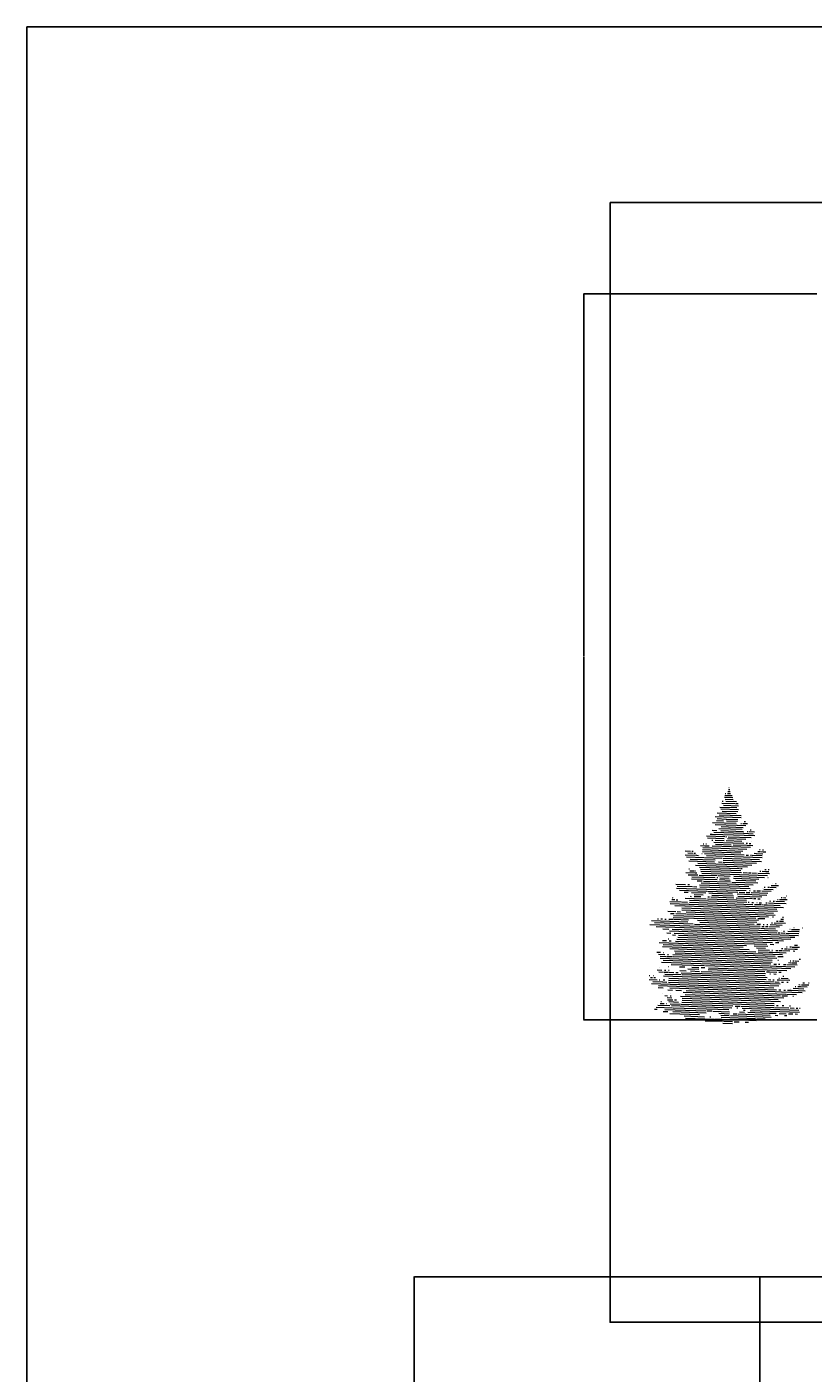
# Model space of a CAD drawing. Units: inches. Extents: x 1770 to 2988, y 1161 to 3221.
# Tile 33 of 44: x 1770 to 2179, y 2520 to 3221. Entities that reach past the tile are written whole.
import ezdxf

# ---------------------------------------------------------------- set-up
doc = ezdxf.new("R2010")
doc.units = ezdxf.units.IN
for name, color, linetype, lineweight in [('A-ANNO-DIMS', 2, 'Continuous', 18), ('A-ANNO-TTLB', 7, 'Continuous', 25), ('trees1', 250, 'Continuous', 13)]:
    doc.layers.add(name, color=color, linetype=linetype, lineweight=lineweight)
doc.styles.get("Standard").update_dxf_attribs({"font": 'arial.ttf'})
doc.dimstyles.get("Standard").update_dxf_attribs({"dimtxt": 0.18, "dimasz": 0.18, "dimexe": 0.18, "dimexo": 0.0625, "dimgap": 0.09, "dimtad": 0, "dimtih": 1, "dimtoh": 1, "dimdec": 4, "dimzin": 0, "dimdsep": 46, "dimtxsty": 'Standard', "dimcen": 0.09, "dimadec": 0, "dimazin": 0, "dimtfac": 1, "dimtdec": 4, "dimtofl": 0, "dimtmove": 0, "dimatfit": 3, "dimfxl": 1, "dimtolj": 1, "dimtzin": 0, "dimarcsym": 0})

# ---------------------------------------------------------------- blocks, each defined once
blk = doc.blocks.new('tree219')
at = {"color": 0}
for p, q in [((17, 2011), (28, 2010)), ((20, 2027), (24, 2027)), ((-38, 1899), (74, 1895)), ((-35, 1915), (-27, 1915)), ((-16, 1947), (53, 1945)), ((-11, 1963), (48, 1961)), ((-10, 1979), (-4, 1979)), ((-8, 1931), (57, 1928)), ((-3, 1914), (85, 1911)), ((11, 1979), (36, 1978)), ((14, 1995), (32, 1994)), ((79, 1895), (98, 1895)), ((-93, 1788), (122, 1780)), ((-75, 1820), (82, 1814)), ((-59, 1803), (124, 1796)), ((-53, 1867), (87, 1863)), ((-45, 1851), (101, 1846)), ((-35, 1834), (94, 1830)), ((-24, 1883), (102, 1878)), ((-116, 1675), (-77, 1674)), ((-114, 1740), (81, 1733)), ((-93, 1723), (86, 1717)), ((-82, 1755), (-23, 1753)), ((-76, 1771), (-2, 1768)), ((-61, 1689), (132, 1683)), ((-44, 1673), (142, 1666)), ((-43, 1705), (140, 1699)), ((2, 1768), (94, 1765)), ((2, 1752), (93, 1749)), ((90, 1717), (161, 1714)), ((121, 1732), (126, 1732)), ((137, 1731), (174, 1730)), ((148, 1747), (159, 1747)), ((171, 1665), (180, 1665)), ((197, 1680), (204, 1680)), ((-192, 1564), (-184, 1564)), ((-169, 1564), (-163, 1563)), ((-164, 1628), (-11, 1623)), ((-155, 1612), (-17, 1607)), ((-132, 1643), (-118, 1643)), ((-120, 1594), (-111, 1594)), ((-117, 1643), (235, 1631)), ((-104, 1659), (141, 1650)), ((-102, 1577), (54, 1572)), ((-93, 1593), (-18, 1591)), ((-89, 1561), (40, 1556)), ((-7, 1623), (3, 1622)), ((0, 1590), (127, 1586)), ((9, 1606), (162, 1601)), ((16, 1622), (204, 1615)), ((57, 1572), (144, 1569)), ((57, 1556), (172, 1552)), ((145, 1650), (222, 1647)), ((165, 1568), (176, 1568)), ((188, 1665), (234, 1663)), ((189, 1567), (203, 1567)), ((206, 1583), (206, 1583)), ((-340, 1505), (-295, 1503)), ((-338, 1472), (-247, 1469)), ((-327, 1456), (-183, 1451)), ((-317, 1488), (-272, 1486)), ((-284, 1503), (-274, 1502)), ((-265, 1486), (-254, 1486)), ((-243, 1469), (-229, 1468)), ((-219, 1468), (-218, 1468)), ((-214, 1549), (-176, 1548)), ((-202, 1484), (-198, 1484)), ((-197, 1516), (136, 1504)), ((-195, 1500), (121, 1489)), ((-193, 1532), (-119, 1529)), ((-180, 1483), (148, 1472)), ((-178, 1450), (-38, 1446)), ((-173, 1548), (-141, 1546)), ((-162, 1466), (297, 1450)), ((-116, 1546), (200, 1535)), ((-116, 1529), (170, 1519)), ((-28, 1445), (275, 1435)), ((163, 1471), (182, 1470)), ((172, 1552), (219, 1550)), ((200, 1470), (207, 1469)), ((213, 1469), (296, 1466)), ((230, 1485), (246, 1484)), ((248, 1484), (300, 1482)), ((261, 1500), (280, 1499)), ((274, 1516), (280, 1516)), ((284, 1499), (304, 1498)), ((299, 1515), (307, 1515)), ((307, 1498), (325, 1498)), ((-308, 1423), (-97, 1415)), ((-308, 1358), (-304, 1358)), ((-302, 1341), (-261, 1340)), ((-298, 1438), (-91, 1431)), ((-254, 1388), (175, 1373)), ((-253, 1340), (-252, 1340)), ((-236, 1404), (212, 1388)), ((-222, 1371), (108, 1359)), ((-213, 1354), (120, 1343)), ((-210, 1338), (126, 1326)), ((-64, 1414), (-34, 1413)), ((-27, 1429), (291, 1418)), ((-26, 1413), (250, 1403)), ((118, 1359), (131, 1359)), ((276, 1337), (284, 1337)), ((297, 1337), (327, 1336)), ((319, 1352), (328, 1352)), ((328, 1336), (351, 1335)), ((344, 1351), (354, 1351)), ((-417, 1232), (-337, 1229)), ((-333, 1326), (-256, 1324)), ((-318, 1229), (-304, 1228)), ((-314, 1309), (-234, 1307)), ((-287, 1276), (-75, 1269)), ((-284, 1292), (-93, 1285)), ((-253, 1323), (-243, 1323)), ((-241, 1258), (-199, 1257)), ((-225, 1306), (-74, 1301)), ((-222, 1225), (185, 1211)), ((-206, 1241), (221, 1226)), ((-203, 1322), (341, 1303)), ((-189, 1256), (35, 1249)), ((-78, 1285), (-69, 1285)), ((-67, 1301), (32, 1297)), ((-57, 1268), (33, 1265)), ((-52, 1284), (24, 1281)), ((46, 1248), (261, 1241)), ((59, 1280), (269, 1273)), ((62, 1296), (315, 1287)), ((78, 1263), (244, 1258)), ((138, 1326), (176, 1325)), ((183, 1324), (203, 1324)), ((212, 1323), (250, 1322)), ((259, 1322), (356, 1318)), ((343, 1286), (344, 1286)), ((380, 1237), (381, 1237)), ((405, 1236), (410, 1236)), ((-447, 1120), (-440, 1119)), ((-412, 1199), (164, 1179)), ((-404, 1215), (-280, 1211)), ((-386, 1182), (-160, 1174)), ((-347, 1165), (-314, 1164)), ((-340, 1116), (-269, 1113)), ((-313, 1131), (-313, 1131)), ((-298, 1131), (-291, 1130)), ((-287, 1163), (-169, 1159)), ((-270, 1211), (-242, 1210)), ((-265, 1129), (-211, 1128)), ((-265, 1113), (-166, 1110)), ((-264, 1146), (-191, 1143)), ((-218, 1209), (197, 1194)), ((-155, 1174), (95, 1166)), ((-151, 1125), (-139, 1125)), ((-143, 1158), (-114, 1157)), ((-128, 1125), (62, 1118)), ((-118, 1141), (60, 1134)), ((-111, 1157), (51, 1151)), ((81, 1117), (215, 1113)), ((89, 1150), (333, 1141)), ((94, 1133), (294, 1126)), ((105, 1165), (154, 1163)), ((165, 1163), (193, 1162)), ((192, 1178), (196, 1178)), ((204, 1162), (342, 1157)), ((225, 1177), (240, 1177)), ((225, 1112), (245, 1112)), ((252, 1176), (281, 1175)), ((260, 1111), (280, 1110)), ((292, 1175), (371, 1172)), ((298, 1191), (299, 1191)), ((309, 1190), (387, 1188)), ((312, 1207), (320, 1206)), ((342, 1205), (354, 1205)), ((359, 1205), (410, 1203)), ((370, 1221), (384, 1220)), ((387, 1220), (431, 1219)), ((453, 1121), (460, 1120)), ((473, 1120), (491, 1119)), ((494, 1135), (496, 1135)), ((-481, 1007), (-417, 1005)), ((-467, 1088), (-372, 1085)), ((-464, 1072), (472, 1039)), ((-448, 1103), (-424, 1103)), ((-424, 1054), (-342, 1051)), ((-414, 1102), (-399, 1102)), ((-405, 1005), (-378, 1004)), ((-368, 1020), (390, 993)), ((-367, 1084), (-320, 1083)), ((-367, 1036), (422, 1008)), ((-340, 1051), (417, 1025)), ((-331, 1002), (404, 976)), ((-304, 1098), (170, 1082)), ((-304, 1082), (220, 1064)), ((-154, 1109), (167, 1098)), ((180, 1082), (188, 1081)), ((212, 1080), (225, 1080)), ((232, 1063), (285, 1062)), ((251, 1079), (255, 1079)), ((270, 1078), (290, 1078)), ((289, 1062), (308, 1061)), ((292, 1094), (294, 1094)), ((311, 1061), (336, 1060)), ((325, 1076), (337, 1076)), ((338, 1060), (444, 1056)), ((348, 1076), (395, 1074)), ((357, 1092), (365, 1091)), ((386, 1091), (398, 1090)), ((395, 1074), (493, 1071)), ((408, 1090), (479, 1087)), ((421, 1105), (429, 1105)), ((440, 1105), (503, 1103)), ((-631, 899), (278, 867)), ((-617, 931), (-316, 921)), ((-593, 914), (-273, 903)), ((-568, 946), (-560, 945)), ((-541, 945), (-527, 944)), ((-508, 943), (-495, 943)), ((-473, 942), (-440, 941)), ((-461, 990), (-429, 989)), ((-439, 957), (-269, 951)), ((-436, 973), (243, 950)), ((-435, 941), (-311, 937)), ((-416, 989), (-334, 986)), ((-328, 986), (348, 962)), ((-266, 951), (265, 933)), ((-261, 902), (280, 884)), ((-238, 934), (253, 917)), ((-219, 917), (231, 901)), ((252, 901), (283, 900)), ((259, 949), (319, 947)), ((305, 899), (312, 899)), ((334, 898), (342, 898)), ((361, 946), (361, 946)), ((362, 897), (460, 893)), ((372, 913), (382, 912)), ((382, 961), (389, 961)), ((396, 912), (488, 909)), ((415, 927), (428, 927)), ((438, 927), (473, 925)), ((450, 942), (471, 942)), ((463, 958), (472, 958)), ((-579, 881), (422, 846)), ((-524, 863), (-474, 861)), ((-490, 829), (-458, 828)), ((-480, 780), (-475, 780)), ((-469, 845), (595, 808)), ((-447, 860), (416, 830)), ((-443, 812), (-418, 811)), ((-429, 827), (516, 794)), ((-408, 778), (382, 750)), ((-401, 794), (422, 765)), ((-394, 810), (531, 778)), ((281, 867), (311, 866)), ((293, 883), (311, 882)), ((314, 866), (406, 863)), ((324, 882), (343, 881)), ((352, 881), (438, 878)), ((425, 830), (445, 829)), ((452, 845), (453, 845)), ((452, 829), (484, 828)), ((471, 844), (480, 844)), ((492, 828), (599, 824)), ((508, 843), (602, 840)), ((522, 794), (564, 793)), ((523, 859), (528, 859)), ((538, 858), (559, 858)), ((557, 874), (560, 874)), ((562, 858), (604, 856)), ((625, 872), (629, 871)), ((-574, 670), (-542, 669)), ((-555, 751), (167, 725)), ((-527, 717), (189, 692)), ((-526, 766), (-493, 765)), ((-522, 733), (138, 710)), ((-518, 668), (-515, 668)), ((-472, 764), (-455, 763)), ((-467, 699), (244, 674)), ((-427, 681), (463, 650)), ((-420, 762), (229, 740)), ((230, 723), (343, 719)), ((234, 739), (334, 736)), ((249, 706), (324, 704)), ((263, 690), (355, 687)), ((263, 674), (346, 671)), ((352, 670), (380, 669)), ((361, 735), (392, 734)), ((375, 686), (381, 686)), ((384, 669), (495, 665)), ((406, 750), (432, 749)), ((408, 685), (425, 684)), ((424, 765), (472, 763)), ((432, 684), (459, 683)), ((456, 699), (465, 699)), ((463, 683), (525, 681)), ((479, 698), (501, 698)), ((496, 714), (502, 714)), ((508, 697), (564, 695)), ((525, 713), (537, 713)), ((544, 712), (605, 710)), ((551, 680), (566, 679)), ((563, 728), (587, 727)), ((569, 695), (588, 695)), ((-560, 654), (-508, 652)), ((-546, 637), (-500, 635)), ((-546, 621), (378, 588)), ((-534, 588), (356, 557)), ((-520, 604), (367, 573)), ((-494, 635), (-445, 633)), ((-484, 651), (-478, 651)), ((-456, 569), (-181, 559)), ((-441, 650), (416, 620)), ((-437, 633), (378, 605)), ((-421, 665), (403, 636)), ((-172, 559), (531, 535)), ((361, 557), (410, 555)), ((391, 572), (413, 571)), ((426, 635), (470, 634)), ((426, 603), (430, 603)), ((431, 570), (442, 570)), ((472, 569), (492, 568)), ((498, 568), (585, 565)), ((513, 584), (531, 583)), ((528, 599), (531, 599)), ((537, 583), (581, 581)), ((549, 599), (560, 598)), ((569, 598), (597, 597)), ((600, 613), (612, 613)), ((-636, 446), (-569, 443)), ((-635, 478), (-632, 478)), ((-624, 461), (-609, 461)), ((-603, 477), (-600, 477)), ((-598, 461), (-585, 460)), ((-570, 524), (-532, 523)), ((-556, 508), (-517, 506)), ((-549, 540), (-548, 540)), ((-517, 474), (329, 444)), ((-512, 506), (-476, 505)), ((-511, 522), (-500, 522)), ((-508, 490), (-373, 485)), ((-477, 521), (-472, 521)), ((-476, 553), (-473, 553)), ((-475, 456), (395, 426)), ((-471, 505), (-434, 503)), ((-415, 503), (-398, 502)), ((-387, 550), (-341, 549)), ((-382, 518), (-330, 516)), ((-373, 501), (320, 477)), ((-364, 485), (337, 460)), ((-316, 532), (-227, 529)), ((-296, 515), (-222, 512)), ((-283, 547), (-227, 545)), ((-207, 544), (-177, 543)), ((-206, 512), (322, 493)), ((-150, 526), (317, 510)), ((-146, 542), (499, 519)), ((331, 509), (356, 508)), ((357, 508), (416, 506)), ((358, 492), (365, 492)), ((393, 491), (410, 490)), ((414, 555), (564, 550)), ((434, 506), (453, 505)), ((434, 457), (439, 457)), ((453, 456), (509, 454)), ((466, 472), (474, 472)), ((-616, 413), (393, 377)), ((-606, 428), (-525, 426)), ((-563, 378), (-520, 377)), ((-559, 394), (413, 360)), ((-553, 443), (-549, 443)), ((-524, 426), (-491, 424)), ((-521, 442), (-507, 441)), ((-482, 359), (-444, 358)), ((-476, 440), (444, 408)), ((-476, 424), (432, 392)), ((-467, 375), (403, 345)), ((-415, 357), (-370, 355)), ((-356, 339), (446, 311)), ((-332, 354), (490, 325)), ((349, 444), (368, 443)), ((384, 442), (396, 442)), ((403, 345), (455, 343)), ((404, 426), (435, 424)), ((419, 441), (435, 441)), ((432, 360), (449, 359)), ((439, 441), (525, 438)), ((454, 424), (473, 423)), ((456, 343), (625, 337)), ((475, 358), (487, 358)), ((500, 422), (510, 422)), ((504, 357), (532, 356)), ((532, 372), (533, 372)), ((534, 356), (651, 352)), ((551, 372), (639, 369)), ((568, 387), (574, 387)), ((590, 387), (610, 386)), ((599, 403), (608, 402)), ((611, 386), (667, 384)), ((621, 402), (653, 401)), ((631, 418), (646, 417)), ((656, 401), (682, 400)), ((677, 416), (683, 416)), ((-566, 233), (-467, 229)), ((-546, 248), (-512, 247)), ((-540, 264), (-535, 264)), ((-527, 328), (-527, 328)), ((-508, 312), (-484, 311)), ((-492, 246), (-491, 246)), ((-488, 295), (-448, 293)), ((-485, 278), (-441, 277)), ((-474, 262), (-435, 260)), ((-464, 310), (-454, 310)), ((-462, 245), (-377, 242)), ((-461, 326), (-461, 326)), ((-451, 229), (46, 211)), ((-433, 260), (-395, 259)), ((-428, 276), (-412, 276)), ((-378, 307), (429, 279)), ((-372, 242), (53, 227)), ((-368, 258), (54, 243)), ((-365, 290), (447, 262)), ((-364, 274), (394, 248)), ((-340, 322), (475, 293)), ((57, 243), (394, 231)), ((73, 226), (111, 225)), ((119, 225), (393, 215)), ((414, 231), (429, 230)), ((459, 310), (506, 309)), ((460, 229), (475, 229)), ((496, 325), (578, 322)), ((520, 227), (530, 227)), ((550, 307), (554, 307)), ((-591, 201), (-570, 200)), ((-579, 217), (-443, 212)), ((-521, 182), (-483, 181)), ((-508, 198), (-167, 186)), ((-466, 164), (-222, 156)), ((-441, 180), (-165, 170)), ((-439, 212), (22, 196)), ((-347, 144), (-181, 138)), ((-337, 127), (-96, 119)), ((-158, 186), (-118, 185)), ((-136, 137), (-128, 136)), ((-111, 184), (27, 179)), ((-92, 119), (-39, 117)), ((-62, 166), (26, 163)), ((-45, 150), (23, 147)), ((-41, 133), (242, 123)), ((-37, 117), (180, 109)), ((35, 147), (369, 135)), ((56, 162), (88, 161)), ((88, 210), (94, 210)), ((96, 161), (361, 152)), ((108, 177), (149, 175)), ((131, 208), (598, 192)), ((143, 192), (155, 191)), ((179, 174), (354, 168)), ((197, 190), (603, 176)), ((251, 123), (320, 121)), ((356, 168), (410, 166)), ((397, 215), (516, 211)), ((402, 150), (424, 149)), ((437, 165), (494, 163)), ((481, 147), (499, 147)), ((513, 162), (549, 161)), ((528, 211), (561, 209)), ((568, 161), (588, 160)), ((575, 209), (589, 208)), ((605, 208), (610, 208)), ((-174, 105), (-32, 100)), ((-29, 84), (52, 81)), ((-23, 100), (50, 98)), ((66, 97), (107, 96)), ((155, 94), (184, 93)), ((191, 109), (246, 107))]:
    blk.add_line(p, q, dxfattribs=at)
blk = doc.blocks.new('*D56')
at = {"layer": 'A-ANNO-DIMS', "color": 0, "lineweight": -2, "transparency": 16777216}
for p, q in [((1971.53, 2506.34), (1971.53, 2570.7)), ((1971.71, 2570.52), (2386.59, 2570.52)), ((2802.26, 2570.52), (2387.38, 2570.52)), ((2802.44, 2506.34), (2802.44, 2570.7))]:
    blk.add_line(p, q, dxfattribs=at)
at = {"layer": 'A-ANNO-DIMS', "color": 0, "transparency": 16777216}
for points in [[(1971.71, 2570.55), (1971.71, 2570.49), (1971.53, 2570.52)], [(2802.26, 2570.55), (2802.26, 2570.49), (2802.44, 2570.52)]]:
    blk.add_solid(points, dxfattribs=at)
at = {"layer": 'Defpoints', "color": 0, "transparency": 16777216}
for p in [(2802.44, 2570.52), (1971.53, 2506.27), (2802.44, 2506.27)]:
    blk.add_point(p, dxfattribs=at)
at = {"layer": 'A-ANNO-DIMS', "color": 0, "transparency": 16777216, "insert": (2386.99, 2570.52), "char_height": 0.18, "attachment_point": 5}
blk.add_mtext('\\A1;830.9', dxfattribs=at)
blk = doc.blocks.new('*D64')
at = {"layer": 'A-ANNO-DIMS', "color": 0, "lineweight": -2, "transparency": 16777216}
for p, q in [((2151.7, 2376.76), (2151.7, 2570.7)), ((2151.88, 2570.52), (2179.09, 2570.52)), ((2207.1, 2570.52), (2179.88, 2570.52)), ((2207.28, 2376.76), (2207.28, 2570.7))]:
    blk.add_line(p, q, dxfattribs=at)
at = {"layer": 'A-ANNO-DIMS', "color": 0, "transparency": 16777216}
for points in [[(2151.88, 2570.55), (2151.88, 2570.49), (2151.7, 2570.52)], [(2207.1, 2570.55), (2207.1, 2570.49), (2207.28, 2570.52)]]:
    blk.add_solid(points, dxfattribs=at)
at = {"layer": 'Defpoints', "color": 0, "transparency": 16777216}
for p in [(2207.28, 2570.52), (2151.7, 2376.7), (2207.28, 2376.7)]:
    blk.add_point(p, dxfattribs=at)
at = {"layer": 'A-ANNO-DIMS', "color": 0, "transparency": 16777216, "insert": (2179.49, 2570.52), "char_height": 0.18, "attachment_point": 5}
blk.add_mtext('\\A1;55.58', dxfattribs=at)
blk = doc.blocks.new('*D79')
at = {"layer": 'A-ANNO-DIMS', "color": 0, "lineweight": -2, "transparency": 16777216}
for p, q in [((2151.7, 1610.26), (2151.7, 2570.7)), ((2151.88, 2570.52), (2177.78, 2570.52)), ((2204.48, 2570.52), (2178.57, 2570.52)), ((2204.66, 1610.26), (2204.66, 2570.7))]:
    blk.add_line(p, q, dxfattribs=at)
at = {"layer": 'A-ANNO-DIMS', "color": 0, "transparency": 16777216}
for points in [[(2151.88, 2570.55), (2151.88, 2570.49), (2151.7, 2570.52)], [(2204.48, 2570.55), (2204.48, 2570.49), (2204.66, 2570.52)]]:
    blk.add_solid(points, dxfattribs=at)
at = {"layer": 'Defpoints', "color": 0, "transparency": 16777216}
for p in [(2204.66, 2570.52), (2151.7, 1610.2), (2204.66, 1610.2)]:
    blk.add_point(p, dxfattribs=at)
at = {"layer": 'A-ANNO-DIMS', "color": 0, "transparency": 16777216, "insert": (2178.18, 2570.52), "char_height": 0.18, "attachment_point": 5}
blk.add_mtext('\\A1;52.96', dxfattribs=at)
blk = doc.blocks.new('*D94')
at = {"layer": 'A-ANNO-DIMS', "color": 0, "lineweight": -2, "transparency": 16777216}
for p, q in [((2181.38, 3082.38), (2059.85, 3082.38)), ((2060.03, 3082.2), (2060.03, 2893.52)), ((2060.03, 2704.48), (2060.03, 2893.16)), ((2181.38, 2704.3), (2059.85, 2704.3))]:
    blk.add_line(p, q, dxfattribs=at)
at = {"layer": 'A-ANNO-DIMS', "color": 0, "transparency": 16777216}
for points in [[(2060, 3082.2), (2060.06, 3082.2), (2060.03, 3082.38)], [(2060, 2704.48), (2060.06, 2704.48), (2060.03, 2704.3)]]:
    blk.add_solid(points, dxfattribs=at)
at = {"layer": 'Defpoints', "color": 0, "transparency": 16777216}
for p in [(2060.03, 3082.38), (2181.44, 3082.38), (2181.44, 2704.3)]:
    blk.add_point(p, dxfattribs=at)
at = {"layer": 'A-ANNO-DIMS', "color": 0, "transparency": 16777216, "insert": (2060.03, 2893.34), "char_height": 0.18, "attachment_point": 5}
blk.add_mtext('\\A1;378.1', dxfattribs=at)

msp = doc.modelspace()

# ---------------------------------------------------------------- linework, layer by layer
at = {"layer": 'A-ANNO-TTLB'}
for points in [[(1769.9155, 3221.2788), (2987.7567, 3221.2788), (2987.7567, 1161.1516), (1769.9155, 1161.1516)], [(2073.6202, 3129.9468), (2769.3644, 3129.9468), (2769.3644, 2546.8952), (2073.6202, 2546.8952)]]:
    msp.add_lwpolyline(points, close=True, dxfattribs=at)

# ---------------------------------------------------------------- block references
at = {"layer": 'trees1', "xscale": 0.063143750371755, "yscale": 0.063143750371755, "zscale": 0.063143750371755}
msp.add_blockref('tree219', (2134.1635, 2697.2516), dxfattribs=at)

# ---------------------------------------------------------------- dimensions: what is measured, and where the dimension line sits
at = {"layer": 'A-ANNO-DIMS'}
dim = msp.add_linear_dim(base=(2060.0309, 3082.3817), p1=(2181.443, 2704.2969), p2=(2181.443, 3082.3817), angle=90, dimstyle='Standard', override={"dimdec": 1, "dimlfac": 1, "dimrnd": 0, "dimzin": 0, "dimdsep": 46, "dimlunit": 2}, dxfattribs=at)
dim.commit()
dim.dimension.update_dxf_attribs({"geometry": '*D94', "text_midpoint": (2060.0309, 2893.3393)})
for base, p1, p2, override, picture, middle in [((2802.4374, 2570.5247), (1971.5344, 2506.2747), (2802.4374, 2506.2747), {"dimdec": 1, "dimlfac": 1, "dimrnd": 0, "dimzin": 0, "dimdsep": 46, "dimlunit": 2}, '*D56', (2386.9859, 2570.5247)), ((2207.2776, 2570.5247), (2151.696, 2376.7021), (2207.2776, 2376.7021), {"dimdec": 2, "dimlfac": 1, "dimrnd": 0, "dimzin": 0, "dimdsep": 46, "dimlunit": 2}, '*D64', (2179.4868, 2570.5247)), ((2204.6568, 2570.5247), (2151.696, 1610.2021), (2204.6568, 1610.2021), {"dimdec": 2, "dimlfac": 1, "dimrnd": 0, "dimzin": 0, "dimdsep": 46, "dimlunit": 2}, '*D79', (2178.1764, 2570.5247))]:
    dim = msp.add_linear_dim(base=base, p1=p1, p2=p2, dimstyle='Standard', override=override, dxfattribs=at)
    dim.commit()
    dim.dimension.update_dxf_attribs({"geometry": picture, "text_midpoint": middle})

doc.saveas('drawing.dxf')
